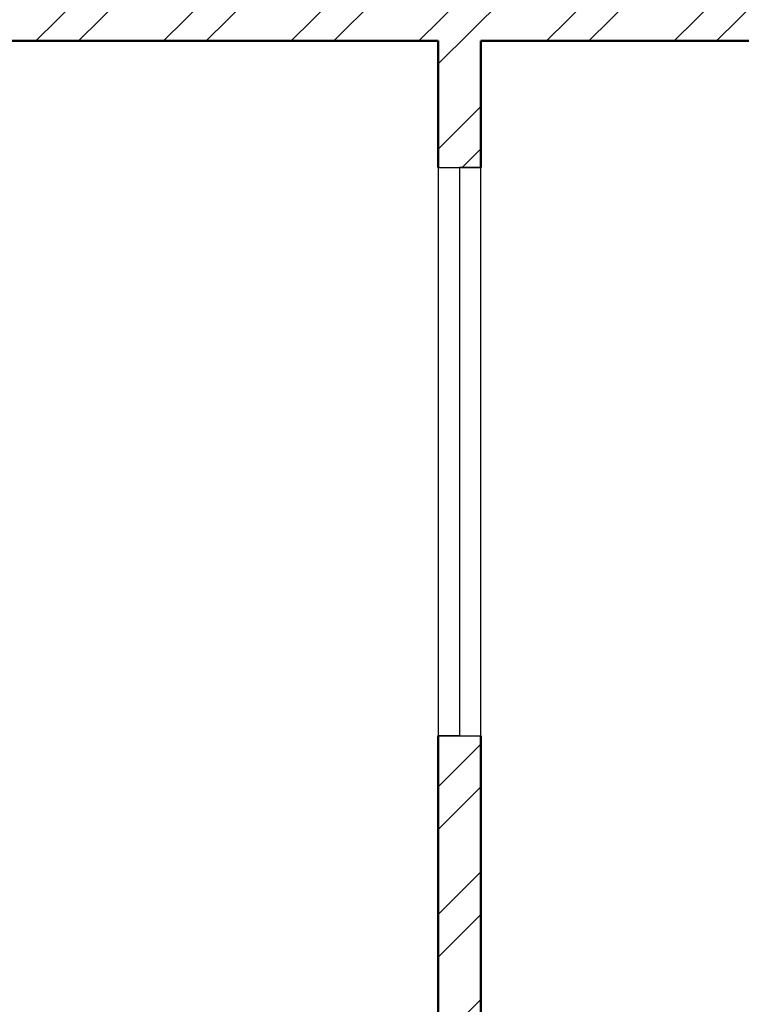
# Model space of a CAD drawing. Units: inches. Extents: x 963 to 2075, y 289 to 2657.
# Tile 94 of 98: x 1809 to 1885, y 2221 to 2325. Entities that reach past the tile are written whole.
import ezdxf

# ---------------------------------------------------------------- set-up
doc = ezdxf.new("R2010")
doc.units = ezdxf.units.IN
for name, color, linetype, lineweight in [('A-GLAZ', 3, 'Continuous', 25), ('A-WALL', 7, 'Continuous', 50), ('A-WALL-PATT', 8, 'Continuous', 13)]:
    doc.layers.add(name, color=color, linetype=linetype, lineweight=lineweight)

msp = doc.modelspace()

# ---------------------------------------------------------------- hatches: boundary and pattern name
at = {"layer": 'A-WALL-PATT'}
h = msp.add_hatch(dxfattribs=at)
h.set_pattern_fill('ANSI32', color=256)
h.paths.add_polyline_path([(1296.92, 2558.32), (1203.92, 2558.32), (1203.92, 2493.82), (1191.53, 2493.82), (1191.53, 2489.32), (1211.06, 2489.32), (1211.06, 2492.02), (1211.06, 2493.82), (1208.42, 2493.82), (1208.42, 2553.82), (1292.42, 2553.82), (1292.42, 2538.86), (1296.92, 2538.86)])
h.paths.add_polyline_path([(1442.42, 2558.32), (1349.42, 2558.32), (1349.42, 2538.94), (1353.92, 2538.94), (1353.92, 2553.82), (1437.92, 2553.82), (1437.92, 2493.82), (1434.54, 2493.82), (1434.54, 2489.32), (1448.31, 2489.32), (1448.31, 2491.57), (1448.31, 2493.82), (1442.42, 2493.82)])
h.paths.add_polyline_path([(1415.55, 2491.57), (1415.55, 2493.82), (1340.94, 2493.82), (1340.94, 2489.32), (1371.92, 2489.32), (1371.92, 2378.32), (1367.6, 2378.32), (1367.6, 2373.82), (1371.92, 2373.82), (1371.92, 2355.19), (1376.42, 2355.19), (1376.42, 2489.32), (1415.55, 2489.32)])
h.paths.add_polyline_path([(1304.94, 2491.57), (1304.94, 2493.82), (1296.92, 2493.82), (1296.92, 2514.86), (1292.42, 2514.86), (1292.42, 2493.82), (1232.81, 2493.82), (1232.81, 2489.32), (1256.42, 2489.32), (1256.42, 2327.32), (1253.71, 2327.32), (1253.71, 2322.82), (1328.42, 2322.82), (1328.42, 2331.15), (1323.92, 2331.15), (1323.92, 2327.32), (1260.92, 2327.32), (1260.92, 2373.82), (1323.92, 2373.82), (1323.92, 2357.81), (1328.42, 2357.81), (1328.42, 2373.82), (1346.01, 2373.82), (1346.01, 2376.07), (1346.01, 2378.32), (1260.92, 2378.32), (1260.92, 2489.32), (1304.94, 2489.32)])
h.paths.add_polyline_path([(1226.65, 2327.32), (1124.42, 2327.32), (1124.42, 2347.45), (1119.92, 2347.45), (1119.92, 2322.82), (1163.42, 2322.82), (1163.42, 2305.43), (1165.67, 2305.43), (1167.92, 2305.43), (1167.92, 2322.82), (1226.65, 2322.82), (1226.65, 2325.07)])
h.paths.add_polyline_path([(1095.92, 2489.32), (1124.42, 2489.32), (1131.53, 2489.32), (1131.53, 2491.57), (1131.53, 2493.82), (1119.92, 2493.82), (1091.42, 2493.82), (1091.42, 2417.32), (1095.92, 2417.32), (1119.92, 2417.32), (1119.92, 2407.45), (1124.42, 2407.45), (1124.42, 2421.82), (1095.92, 2421.82)])
h.paths.add_polyline_path([(1512.92, 2558.32), (1508.42, 2558.32), (1508.42, 2493.82), (1503.4, 2493.82), (1503.4, 2489.32), (1508.42, 2489.32), (1508.42, 2327.32), (1376.42, 2327.32), (1376.42, 2330.27), (1371.92, 2330.27), (1371.92, 2298.74), (1376.42, 2298.74), (1376.42, 2322.82), (1508.42, 2322.82), (1508.42, 2165.32), (1504.26, 2165.32), (1504.26, 2160.82), (1508.42, 2160.82), (1508.42, 2108.32), (1512.92, 2108.32), (1512.92, 2160.82), (1516.18, 2160.82), (1516.18, 2163.07), (1516.18, 2165.32), (1512.92, 2165.32), (1512.92, 2322.82), (1644.92, 2322.82), (1644.92, 2298.74), (1649.42, 2298.74), (1649.42, 2322.82), (1649.42, 2330.94), (1647.17, 2330.94), (1644.92, 2330.94), (1644.92, 2327.32), (1512.92, 2327.32), (1512.92, 2489.32), (1516.76, 2489.32), (1516.76, 2491.57), (1516.76, 2493.82), (1512.92, 2493.82)])
h.paths.add_polyline_path([(1671.92, 2558.32), (1578.92, 2558.32), (1578.92, 2493.82), (1573.53, 2493.82), (1573.53, 2489.32), (1586.54, 2489.32), (1586.54, 2491.57), (1586.54, 2493.82), (1583.42, 2493.82), (1583.42, 2553.82), (1667.42, 2553.82), (1667.42, 2541.11), (1671.92, 2541.11)])
h.paths.add_polyline_path([(1681.26, 2493.82), (1671.92, 2493.82), (1671.92, 2517.11), (1667.42, 2517.11), (1667.42, 2493.82), (1610.22, 2493.82), (1610.22, 2489.32), (1644.92, 2489.32), (1644.92, 2357.87), (1649.42, 2357.87), (1649.42, 2373.82), (1652.2, 2373.82), (1652.2, 2375.83), (1652.2, 2378.32), (1649.42, 2378.32), (1649.42, 2489.32), (1681.26, 2489.32), (1681.26, 2491.57)])
h.paths.add_polyline_path([(1821.92, 2558.32), (1728.92, 2558.32), (1728.92, 2541), (1733.42, 2541), (1733.42, 2553.82), (1817.42, 2553.82), (1817.42, 2493.82), (1813.51, 2493.82), (1813.51, 2489.32), (1830.08, 2489.32), (1830.08, 2491.57), (1830.08, 2493.82), (1821.92, 2493.82)])
h.paths.add_polyline_path([(1794.24, 2493.82), (1717.26, 2493.82), (1717.26, 2489.32), (1760.42, 2489.32), (1760.42, 2378.32), (1674.4, 2378.32), (1674.4, 2373.82), (1692.92, 2373.82), (1692.92, 2356.95), (1697.42, 2356.95), (1697.42, 2373.82), (1760.42, 2373.82), (1760.42, 2327.32), (1697.42, 2327.32), (1697.42, 2333.34), (1692.92, 2333.34), (1692.92, 2322.82), (1768.04, 2322.82), (1768.04, 2325.07), (1768.04, 2327.32), (1764.92, 2327.32), (1764.92, 2489.32), (1794.24, 2489.32)])
h.paths.add_polyline_path([(1733.42, 2517), (1728.92, 2517), (1728.92, 2493.82), (1733.42, 2493.82)], flags=17)
h.paths.add_polyline_path([(1929.92, 2493.82), (1890.08, 2493.82), (1890.08, 2489.32), (1896.92, 2489.32), (1925.42, 2489.32), (1925.42, 2421.82), (1896.92, 2421.82), (1896.92, 2408.32), (1901.42, 2408.32), (1901.42, 2417.32), (1925.42, 2417.32), (1929.92, 2417.32)])
h.paths.add_polyline_path([(1901.42, 2348.32), (1896.92, 2348.32), (1896.92, 2327.32), (1800.42, 2327.32), (1800.42, 2322.82), (1853.42, 2322.82), (1853.42, 2309.45), (1857.92, 2309.45), (1857.92, 2322.82), (1901.42, 2322.82)])
h.paths.add_polyline_path([(1857.92, 2249.45), (1853.42, 2249.45), (1853.42, 2214.82), (1686.31, 2214.82), (1686.31, 2210.32), (1853.42, 2210.32), (1853.42, 2202.13), (1857.92, 2202.13), (1857.92, 2210.32)])
h.paths.add_polyline_path([(1857.92, 2142.13), (1853.42, 2142.13), (1853.42, 2115.42), (1841.42, 2115.42), (1841.42, 2088.53), (1841.42, 2046.95), (1845.92, 2046.95), (1845.92, 2110.92), (1905.92, 2110.92), (1905.92, 2092.52), (1910.42, 2092.52), (1910.42, 2115.42), (1857.92, 2115.42)])
h.paths.add_polyline_path([(1532.44, 1482.34), (1573.46, 1482.34), (1573.46, 1501), (1532.44, 1501)], flags=9)
h.paths.add_polyline_path([(1438.66, 1486.3), (1479.68, 1486.3), (1479.68, 1504.96), (1438.66, 1504.96)], flags=9)
h.paths.add_polyline_path([(1411.22, 1365.31), (1659.14, 1365.31), (1659.14, 1402.4), (1411.22, 1402.4)], flags=9)
h.paths.add_polyline_path([(1185.67, 2296.3), (1248.16, 2296.3), (1248.16, 2314.95), (1185.67, 2314.95)], flags=9)
h.paths.add_polyline_path([(1177.31, 2187.35), (1216.15, 2187.35), (1216.15, 2206.01), (1177.31, 2206.01)], flags=9)
h.paths.add_polyline_path([(1295.1, 1602.08), (1328.26, 1602.08), (1328.26, 1620.74), (1295.1, 1620.74)], flags=9)
h.paths.add_polyline_path([(1525.13, 2005.99), (1558.39, 2005.99), (1558.39, 2024.65), (1525.13, 2024.65)], flags=9)
h.paths.add_polyline_path([(1459.61, 1977.13), (1472.19, 1977.13), (1472.19, 1987.43), (1459.61, 1987.43)], flags=9)
h.paths.add_polyline_path([(1467.81, 2053.68), (1480.02, 2053.68), (1480.02, 2063.98), (1467.81, 2063.98)], flags=9)
h.paths.add_polyline_path([(1555.18, 2119.02), (1584.56, 2119.02), (1584.56, 2137.68), (1555.18, 2137.68)], flags=25)
h.paths.add_polyline_path([(1405.39, 2115.29), (1444.48, 2115.29), (1444.48, 2133.95), (1405.39, 2133.95)], flags=25)
h.paths.add_polyline_path([(1698.48, 2004.26), (1727.69, 2004.26), (1727.69, 2022.92), (1698.48, 2022.92)], flags=9)
h.paths.add_polyline_path([(1612.16, 1972.86), (1629.02, 1972.86), (1629.02, 1983.16), (1612.16, 1983.16)], flags=9)
h.paths.add_polyline_path([(1608.29, 2060.04), (1625.15, 2060.04), (1625.15, 2070.34), (1608.29, 2070.34)], flags=9)
h.paths.add_polyline_path([(1527.95, 1684.4), (1566.79, 1684.4), (1566.79, 1703.06), (1527.95, 1703.06)], flags=9)
h.paths.add_polyline_path([(1422.79, 1683.59), (1461.63, 1683.59), (1461.63, 1702.25), (1422.79, 1702.25)], flags=9)
h.paths.add_polyline_path([(1531.26, 1732.46), (1574.01, 1732.46), (1574.01, 1751.12), (1531.26, 1751.12)], flags=9)
h.paths.add_polyline_path([(1402.87, 1732.85), (1439.8, 1732.85), (1439.8, 1751.5), (1402.87, 1751.5)], flags=9)
h.paths.add_polyline_path([(1243.12, 1923.13), (1281.96, 1923.13), (1281.96, 1941.79), (1243.12, 1941.79)], flags=9)
h.paths.add_polyline_path([(1181.75, 1792.27), (1244.24, 1792.27), (1244.24, 1810.93), (1181.75, 1810.93)], flags=9)
h.paths.add_polyline_path([(1265.82, 1670.3), (1316.07, 1670.3), (1316.07, 1688.96), (1265.82, 1688.96)], flags=9)
h.paths.add_polyline_path([(1140.26, 1676.05), (1179.1, 1676.05), (1179.1, 1694.71), (1140.26, 1694.71)], flags=9)
h.paths.add_polyline_path([(1107.49, 1490.89), (1143.37, 1490.89), (1143.37, 1509.55), (1107.49, 1509.55)], flags=9)
h.paths.add_polyline_path([(1217.58, 1483.9), (1246.74, 1483.9), (1246.74, 1502.56), (1217.58, 1502.56)], flags=9)
h.paths.add_polyline_path([(1389.21, 1486.92), (1418.37, 1486.92), (1418.37, 1505.58), (1389.21, 1505.58)], flags=9)
h.paths.add_polyline_path([(1672.21, 1602.08), (1705.37, 1602.08), (1705.37, 1620.74), (1672.21, 1620.74)], flags=9)
h.paths.add_polyline_path([(1752.08, 1522.64), (1781.24, 1522.64), (1781.24, 1541.3), (1752.08, 1541.3)], flags=9)
h.paths.add_polyline_path([(1848.27, 1491.26), (1884.16, 1491.26), (1884.16, 1509.92), (1848.27, 1509.92)], flags=9)
h.paths.add_polyline_path([(1822.47, 1685.62), (1861.31, 1685.62), (1861.31, 1704.28), (1822.47, 1704.28)], flags=9)
h.paths.add_polyline_path([(1713.19, 1672.23), (1763.44, 1672.23), (1763.44, 1690.89), (1713.19, 1690.89)], flags=9)
h.paths.add_polyline_path([(1736.62, 1790.58), (1799.11, 1790.58), (1799.11, 1809.24), (1736.62, 1809.24)], flags=9)
h.paths.add_polyline_path([(1691.49, 1916.36), (1730.33, 1916.36), (1730.33, 1935.01), (1691.49, 1935.01)], flags=9)
h.paths.add_polyline_path([(1764.87, 1973.92), (1794.31, 1973.92), (1794.31, 1992.58), (1764.87, 1992.58)], flags=9)
h.paths.add_polyline_path([(1767.85, 2034.02), (1797.29, 2034.02), (1797.29, 2052.67), (1767.85, 2052.67)], flags=9)
h.paths.add_polyline_path([(1851.59, 2060.33), (1880.75, 2060.33), (1880.75, 2078.99), (1851.59, 2078.99)], flags=25)
h.paths.add_polyline_path([(1688.49, 2086.87), (1727.33, 2086.87), (1727.33, 2105.53), (1688.49, 2105.53)], flags=9)
h.paths.add_polyline_path([(1537.74, 2293.58), (1580.49, 2293.58), (1580.49, 2312.24), (1537.74, 2312.24)], flags=25)
h.paths.add_polyline_path([(1425.59, 2296.11), (1468.34, 2296.11), (1468.34, 2314.77), (1425.59, 2314.77)], flags=25)
h.paths.add_polyline_path([(1278.52, 2004.18), (1307.72, 2004.18), (1307.72, 2022.84), (1278.52, 2022.84)], flags=9)
h.paths.add_polyline_path([(1193.28, 1973.63), (1222.72, 1973.63), (1222.72, 1992.29), (1193.28, 1992.29)], flags=9)
h.paths.add_polyline_path([(1192.41, 2040.58), (1221.84, 2040.58), (1221.84, 2059.23), (1192.41, 2059.23)], flags=9)
h.paths.add_polyline_path([(1130.6, 1951.39), (1159.76, 1951.39), (1159.76, 1970.05), (1130.6, 1970.05)], flags=9)
h.paths.add_polyline_path([(1132.83, 2052.49), (1161.98, 2052.49), (1161.98, 2071.15), (1132.83, 2071.15)], flags=9)
h.paths.add_polyline_path([(1265.13, 2334.62), (1315.38, 2334.62), (1315.38, 2353.28), (1265.13, 2353.28)], flags=25)
h.paths.add_polyline_path([(1136.74, 2330.79), (1175.58, 2330.79), (1175.58, 2349.44), (1136.74, 2349.44)], flags=9)
h.paths.add_polyline_path([(1287.42, 2417.2), (1320.58, 2417.2), (1320.58, 2435.86), (1287.42, 2435.86)], flags=25)
h.paths.add_polyline_path([(1430.99, 2329.16), (1469.83, 2329.16), (1469.83, 2347.82), (1430.99, 2347.82)], flags=25)
h.paths.add_polyline_path([(1525.42, 2329.21), (1564.26, 2329.21), (1564.26, 2347.87), (1525.42, 2347.87)], flags=25)
h.paths.add_polyline_path([(1684.52, 2382.8), (1717.68, 2382.8), (1717.68, 2401.46), (1684.52, 2401.46)], flags=25)
h.paths.add_polyline_path([(1704.81, 2340.29), (1755.05, 2340.29), (1755.05, 2358.95), (1704.81, 2358.95)], flags=25)
h.paths.add_polyline_path([(1694.11, 2287.76), (1756.6, 2287.76), (1756.6, 2306.41), (1694.11, 2306.41)], flags=9)
h.paths.add_polyline_path([(1815.78, 2329.86), (1854.62, 2329.86), (1854.62, 2348.52), (1815.78, 2348.52)], flags=9)
h.paths.add_polyline_path([(1842.87, 2514.26), (1878.76, 2514.26), (1878.76, 2532.91), (1842.87, 2532.91)], flags=9)
h.paths.add_polyline_path([(1769.51, 2531.45), (1798.67, 2531.45), (1798.67, 2550.1), (1769.51, 2550.1)], flags=25)
h.paths.add_polyline_path([(1594.77, 2518.47), (1623.93, 2518.47), (1623.93, 2537.13), (1594.77, 2537.13)], flags=25)
h.paths.add_polyline_path([(1520.72, 2516.18), (1556.61, 2516.18), (1556.61, 2534.84), (1520.72, 2534.84)], flags=25)
h.paths.add_polyline_path([(1464.46, 2516.69), (1500.34, 2516.69), (1500.34, 2535.35), (1464.46, 2535.35)], flags=25)
h.paths.add_polyline_path([(1365.7, 2528.97), (1394.85, 2528.97), (1394.85, 2547.63), (1365.7, 2547.63)], flags=25)
h.paths.add_polyline_path([(1222.84, 2516.23), (1252, 2516.23), (1252, 2534.89), (1222.84, 2534.89)], flags=25)
h.paths.add_polyline_path([(1104.55, 2509.6), (1140.43, 2509.6), (1140.43, 2528.26), (1104.55, 2528.26)], flags=9)

# ---------------------------------------------------------------- linework, layer by layer
at = {"layer": 'A-GLAZ'}
for p, q in [((1853.42, 2309.45), (1857.92, 2309.45)), ((1853.42, 2309.45), (1853.42, 2249.45)), ((1857.92, 2309.45), (1855.67, 2309.45)), ((1855.67, 2309.45), (1855.67, 2249.45)), ((1857.92, 2249.45), (1857.92, 2309.45)), ((1855.67, 2249.45), (1853.42, 2249.45)), ((1853.42, 2249.45), (1857.92, 2249.45))]:
    msp.add_line(p, q, dxfattribs=at)
at = {"layer": 'A-WALL'}
for p, q in [((1800.42, 2322.82), (1853.42, 2322.82)), ((1853.42, 2322.82), (1853.42, 2309.45)), ((1857.92, 2322.82), (1857.92, 2309.45)), ((1857.92, 2322.82), (1901.42, 2322.82)), ((1853.42, 2249.45), (1853.42, 2214.82)), ((1857.92, 2249.45), (1857.92, 2210.32))]:
    msp.add_line(p, q, dxfattribs=at)

doc.saveas('drawing.dxf')
